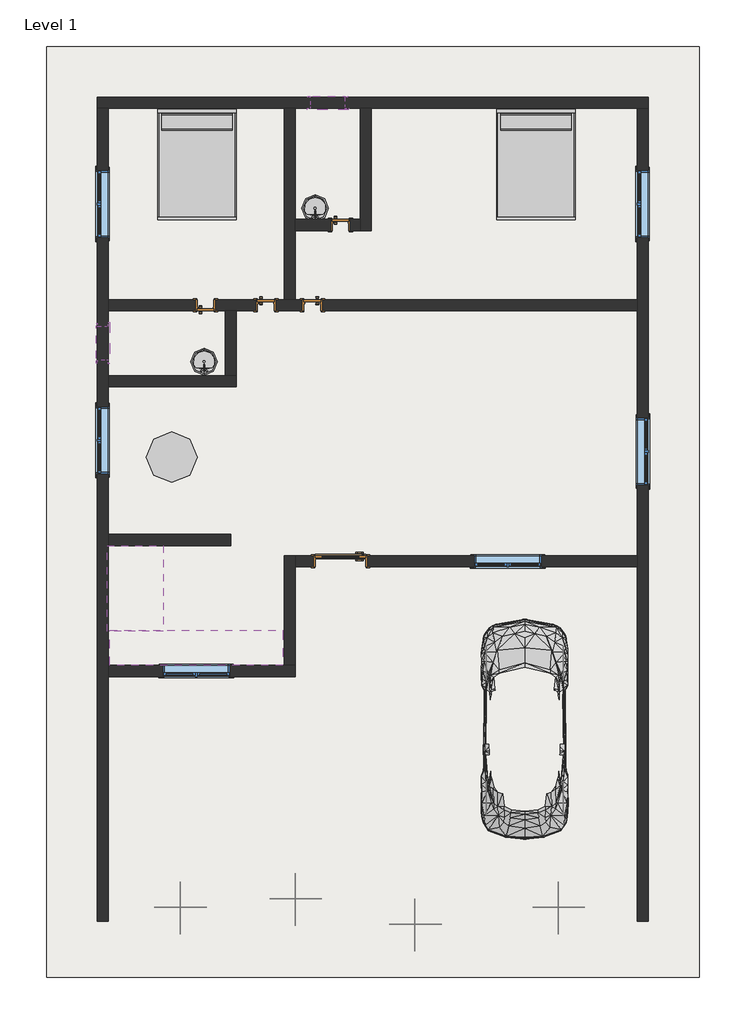
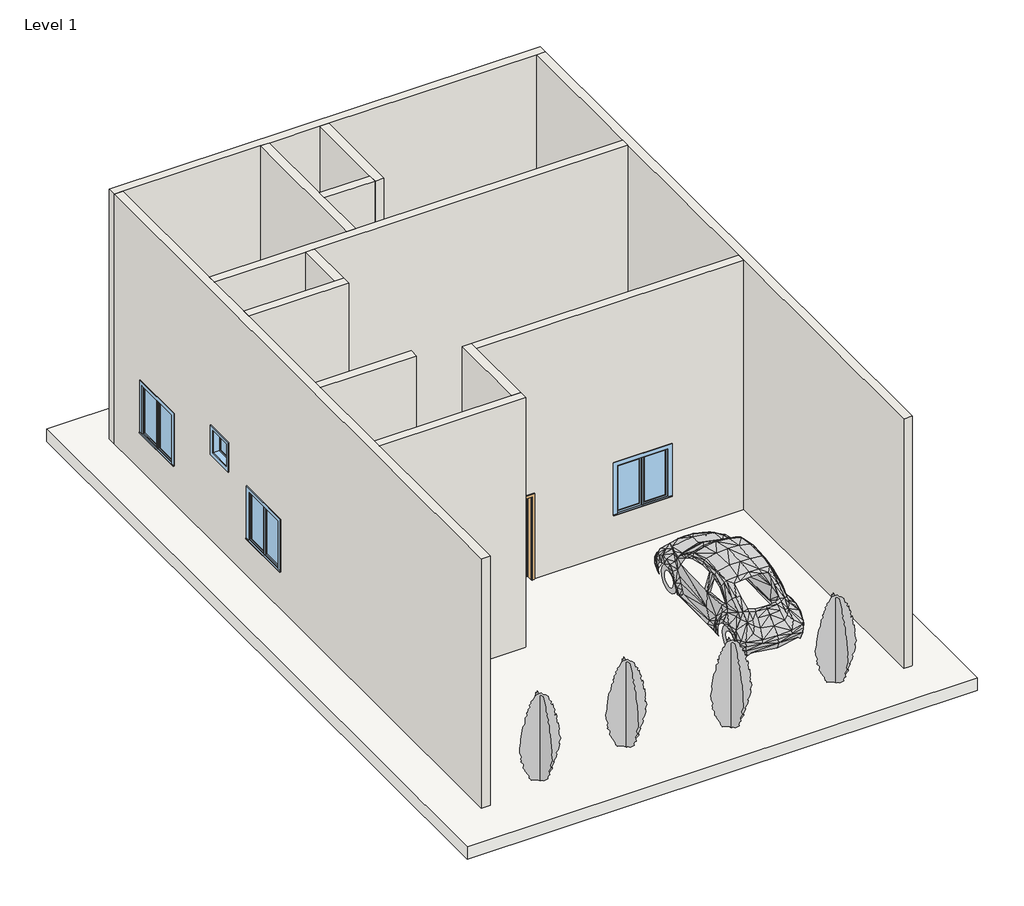
# One storey, incomplete: 13 walls, 8 windows, 5 doors, 5 furniture elements, 4 geographic elements, 2 flow terminals, 1 proxy, 1 slab.
"""IFC4 building model written with IfcOpenShell, lengths in millimetres."""

from ifc_helpers import new_model, si_unit, frame, origin, origin_with_axes, place, context, project, spatial, polyline, outline, extrude, faceted_brep, transform, mapped, element, save
from components import rpc_beetle_rpc_beetle_3ce7ba48, door_1768e003, door_5a382651, door_6ef897ee, door_21b72c96, door_b2d2822a, flow_terminal_d49f872f, furniture_096e7f55, furniture_ac307b45, furniture_905aceb5, furniture_cbbb8910, rpc_tree_conifer_chinese_juniper_7_1b9786cd, window_0862ab64, window_e41d21a6

model = new_model("IFC4")

# Units and contexts
model_context = context("Model", 3, world=origin())
ifc_project = project(units=[si_unit("LENGTHUNIT", "METRE", prefix="MILLI")], contexts=[model_context])

# Site, building, storey
site = spatial("IfcSite", under=ifc_project)
building = spatial("IfcBuilding", under=site)
storey = spatial("IfcBuildingStorey", under=building, Name="Level 1", Elevation=0.0)

# Proxy
placement = place(None, origin())
rpc_beetle_rpc_beetle_shape = rpc_beetle_rpc_beetle_3ce7ba48(model_context)
element("IfcBuildingElementProxy", 1, Name="RPC Beetle : RPC Beetle", ObjectType="RPC Beetle : RPC Beetle", at=placement, inside=storey, context=model_context, shape_type="MappedRepresentation", body=[
    mapped(rpc_beetle_rpc_beetle_shape, transform((-1661.472393, 1425.4293124, 0.0), x_axis=(1.0, 0.0, 0.0), y_axis=(0.0, 1.0, 0.0), z_axis=(0.0, 0.0, 1.0))),
])

# Doors
door_shape = door_1768e003(model_context)
element("IfcDoor", 2, ObjectType="36\" x 80\"", at=placement, inside=storey, context=model_context, shape_type="MappedRepresentation", body=[
    mapped(door_shape, transform((-4988.872393, 5695.8043124, 0.0), x_axis=(1.0, 0.0, 0.0), y_axis=(0.0, 1.0, 0.0), z_axis=(0.0, 0.0, 1.0))),
])
door_2_shape = door_5a382651(model_context)
element("IfcDoor", 3, ObjectType="Door-Interior-Single-5_Panel_Vert-Wood : 12\" x 80\"", at=placement, inside=storey, context=model_context, shape_type="MappedRepresentation", body=[
    mapped(door_2_shape, transform((-6335.072393, 10318.6043124, 0.0), x_axis=(1.0, 0.0, 0.0), y_axis=(0.0, 1.0, 0.0), z_axis=(0.0, 0.0, 1.0))),
])
door_3_shape = door_6ef897ee(model_context)
element("IfcDoor", 4, ObjectType="Door-Interior-Single-5_Panel_Vert-Wood : 12\" x 80\"", at=placement, inside=storey, context=model_context, shape_type="MappedRepresentation", body=[
    mapped(door_3_shape, transform((-5496.872393, 10318.6043124, 0.0), x_axis=(-1.0, 0.0, 0.0), y_axis=(0.0, -1.0, 0.0), z_axis=(0.0, 0.0, 1.0))),
])
door_4_shape = door_21b72c96(model_context)
element("IfcDoor", 5, ObjectType="Door-Interior-Single-Flush_Panel-Wood : 12\" x 80\"", at=placement, inside=storey, context=model_context, shape_type="MappedRepresentation", body=[
    mapped(door_4_shape, transform((-7427.272393, 10312.2543124, 0.0), x_axis=(1.0, 0.0, 0.0), y_axis=(0.0, 1.0, 0.0), z_axis=(0.0, 0.0, 1.0))),
])
door_5_shape = door_b2d2822a(model_context)
element("IfcDoor", 6, ObjectType="Door-Interior-Single-Flush_Panel-Wood : 12\" x 80\"", at=placement, inside=storey, context=model_context, shape_type="MappedRepresentation", body=[
    mapped(door_5_shape, transform((-4988.872393, 11766.4043124, 0.0), x_axis=(1.0, 0.0, 0.0), y_axis=(0.0, 1.0, 0.0), z_axis=(0.0, 0.0, 1.0))),
])

# Flow terminals
flow_terminal_shape = flow_terminal_d49f872f(model_context)
element("IfcFlowTerminal", 7, ObjectType="Sink Vanity-Round : 19\" x 19\"", at=placement, inside=storey, context=model_context, shape_type="MappedRepresentation", body=[
    mapped(flow_terminal_shape, transform((-7356.0206524, 9381.7686876, 0.0), x_axis=(-1.0000000000000004, 0.0, 0.0), y_axis=(0.0, -1.0000000000000004, 0.0), z_axis=(0.0, 0.0, 1.0))),
])
element("IfcFlowTerminal", 8, ObjectType="Sink Vanity-Round : 19\" x 19\"", at=placement, inside=storey, context=model_context, shape_type="MappedRepresentation", body=[
    mapped(flow_terminal_shape, transform((-5349.4206524, 12154.1555452, 0.0), x_axis=(-1.0, 0.0, 0.0), y_axis=(0.0, -1.0, 0.0), z_axis=(0.0, 0.0, 1.0))),
])

# Furniture
furniture_shape = furniture_096e7f55(model_context)
element("IfcFurniture", 9, ObjectType="Bed-Shaker : Double 56\" x 78\"", at=placement, inside=storey, context=model_context, shape_type="MappedRepresentation", body=[
    mapped(furniture_shape, transform((-7560.622393, 13846.0293124, 0.0), x_axis=(1.0, 0.0, 0.0), y_axis=(0.0, 1.0, 0.0), z_axis=(0.0, 0.0, 1.0))),
])
element("IfcFurniture", 10, ObjectType="Bed-Shaker : Double 56\" x 78\"", at=placement, inside=storey, context=model_context, shape_type="MappedRepresentation", body=[
    mapped(furniture_shape, transform((-1439.222393, 13846.0293124, 0.0), x_axis=(1.0, 0.0, 0.0), y_axis=(0.0, 1.0, 0.0), z_axis=(0.0, 0.0, 1.0))),
])
furniture_2_shape = furniture_ac307b45(model_context)
element("IfcFurniture", 11, ObjectType="Counter Top-Island : 48\" Depth", at=placement, inside=storey, context=model_context, shape_type="MappedRepresentation", body=[
    mapped(furniture_2_shape, transform((-9179.872393, 5629.4416075, 914.4), x_axis=(0.0, 1.0000000000000002, 0.0), y_axis=(-1.0000000000000002, 0.0, 0.0), z_axis=(0.0, 0.0, 1.0))),
])
furniture_3_shape = furniture_905aceb5(model_context)
element("IfcFurniture", 12, ObjectType="Table-Dining Round w Chairs : 36\" Diameter", at=placement, inside=storey, context=model_context, shape_type="MappedRepresentation", body=[
    mapped(furniture_3_shape, transform((-8140.5543602, 7757.108001, 0.0), x_axis=(1.0, 0.0, 0.0), y_axis=(0.0, 1.0, 0.0), z_axis=(0.0, 0.0, 1.0))),
])
furniture_4_shape = furniture_cbbb8910(model_context)
element("IfcFurniture", 13, ObjectType="Vanity Counter Top w Square Sink Hole : 24\" Depth", at=placement, inside=storey, context=model_context, shape_type="MappedRepresentation", body=[
    mapped(furniture_4_shape, transform((-7885.7560093, 4448.0293124, 914.4), x_axis=(1.0, 0.0, 0.0), y_axis=(0.0, 1.0, 0.0), z_axis=(0.0, 0.0, 1.0))),
])

# Geographic elements
rpc_tree_conifer_chinese_juniper_7_shape = rpc_tree_conifer_chinese_juniper_7_1b9786cd(model_context)
element("IfcGeographicElement", 14, ObjectType="RPC Tree - Conifer : Chinese Juniper - 7'", at=placement, inside=storey, context=model_context, shape_type="MappedRepresentation", body=[
    mapped(rpc_tree_conifer_chinese_juniper_7_shape, transform((-1052.0690641, -555.7706876, 0.0), x_axis=(1.0, 0.0, 0.0), y_axis=(0.0, 1.0, 0.0), z_axis=(0.0, 0.0, 1.0))),
])
element("IfcGeographicElement", 15, ObjectType="RPC Tree - Conifer : Chinese Juniper - 7'", at=placement, inside=storey, context=model_context, shape_type="MappedRepresentation", body=[
    mapped(rpc_tree_conifer_chinese_juniper_7_shape, transform((-3642.8690641, -860.5706876, 0.0), x_axis=(1.0, 0.0, 0.0), y_axis=(0.0, 1.0, 0.0), z_axis=(0.0, 0.0, 1.0))),
])
element("IfcGeographicElement", 16, ObjectType="RPC Tree - Conifer : Chinese Juniper - 7'", at=placement, inside=storey, context=model_context, shape_type="MappedRepresentation", body=[
    mapped(rpc_tree_conifer_chinese_juniper_7_shape, transform((-7884.6690641, -555.7706876, 0.0), x_axis=(1.0, 0.0, 0.0), y_axis=(0.0, 1.0, 0.0), z_axis=(0.0, 0.0, 1.0))),
])
element("IfcGeographicElement", 17, ObjectType="RPC Tree - Conifer : Chinese Juniper - 7'", at=placement, inside=storey, context=model_context, shape_type="MappedRepresentation", body=[
    mapped(rpc_tree_conifer_chinese_juniper_7_shape, transform((-5801.8690641, -403.3706876, 0.0), x_axis=(1.0, 0.0, 0.0), y_axis=(0.0, 1.0, 0.0), z_axis=(0.0, 0.0, 1.0))),
])

# Slab
element("IfcSlab", 18, ObjectType="Generic - 12\"", at=placement, inside=storey, context=model_context, shape_type="SweptSolid", body=[
    extrude(outline(polyline([(-10297.472393, 14989.0293124), (1488.127607, 14989.0293124), (1488.127607, -1825.7706876), (-10297.472393, -1825.7706876), (-10297.472393, 14989.0293124)])), frame((0.0, 0.0, -304.8), z_axis=(0.0, 0.0, 1.0), x_axis=(1.0, 0.0, 0.0)), (0.0, 0.0, 1.0), 304.8),
])

# Walls
element("IfcWall", 19, ObjectType="Generic - 8\"", at=placement, inside=storey, context=model_context, shape_type="Brep", body=[
    faceted_brep([(-9383.072393, 13871.4293124, 0.0), (-9179.872393, 13871.4293124, 0.0), (-6004.872393, 13871.4293124, 0.0), (-5801.672393, 13871.4293124, 0.0), (-4633.272393, 13871.4293124, 0.0), (-4430.072393, 13871.4293124, 0.0), (370.527607, 13871.4293124, 0.0), (573.727607, 13871.4293124, 0.0), (573.727607, 13871.4293124, 6096.0), (370.527607, 13871.4293124, 6096.0), (-4430.072393, 13871.4293124, 6096.0), (-4633.272393, 13871.4293124, 6096.0), (-5801.672393, 13871.4293124, 6096.0), (-6004.872393, 13871.4293124, 6096.0), (-9179.872393, 13871.4293124, 6096.0), (-9383.072393, 13871.4293124, 6096.0), (-5522.272393, 13871.4293124, 2768.6), (-4912.672393, 13871.4293124, 2768.6), (-4912.672393, 13871.4293124, 2159.0), (-5522.272393, 13871.4293124, 2159.0), (-9383.072393, 14074.6293124, 0.0), (-9383.072393, 14074.6293124, 6096.0), (573.727607, 14074.6293124, 6096.0), (573.727607, 14074.6293124, 0.0), (-5522.272393, 14074.6293124, 2768.6), (-5522.272393, 14074.6293124, 2159.0), (-4912.672393, 14074.6293124, 2159.0), (-4912.672393, 14074.6293124, 2768.6)], [[[0, 1, 2, 3, 4, 5, 6, 7, 8, 9, 10, 11, 12, 13, 14, 15], [16, 17, 18, 19]], [[20, 21, 22, 23], [24, 25, 26, 27]], [[7, 6, 5, 4, 3, 2, 1, 0, 20, 23]], [[15, 14, 13, 12, 11, 10, 9, 8, 22, 21]], [[8, 7, 23, 22]], [[0, 15, 21, 20]], [[25, 24, 16, 19]], [[26, 25, 19, 18]], [[27, 26, 18, 17]], [[24, 27, 17, 16]]]),
])
element("IfcWall", 20, ObjectType="Generic - 8\"", at=placement, inside=storey, context=model_context, shape_type="Brep", body=[
    faceted_brep([(370.527607, 13871.4293124, 0.0), (370.527607, 10417.0293124, 0.0), (370.527607, 10213.8293124, 0.0), (370.527607, 5794.2293124, 0.0), (370.527607, 5591.0293124, 0.0), (370.527607, -809.7706876, 0.0), (370.527607, -809.7706876, 6096.0), (370.527607, 5591.0293124, 6096.0), (370.527607, 5794.2293124, 6096.0), (370.527607, 10213.8293124, 6096.0), (370.527607, 10417.0293124, 6096.0), (370.527607, 13871.4293124, 6096.0), (370.527607, 12753.8293124, 2133.6), (370.527607, 11534.6293124, 2133.6), (370.527607, 11534.6293124, 914.4), (370.527607, 12753.8293124, 914.4), (370.527607, 7064.2293124, 2133.6), (370.527607, 7064.2293124, 914.4), (370.527607, 8283.4293124, 914.4), (370.527607, 8283.4293124, 2133.6), (573.727607, 13871.4293124, 0.0), (573.727607, 13871.4293124, 6096.0), (573.727607, -809.7706876, 6096.0), (573.727607, -809.7706876, 0.0), (573.727607, 12753.8293124, 2133.6), (573.727607, 12753.8293124, 914.4), (573.727607, 11534.6293124, 914.4), (573.727607, 11534.6293124, 2133.6), (573.727607, 7064.2293124, 2133.6), (573.727607, 8283.4293124, 2133.6), (573.727607, 8283.4293124, 914.4), (573.727607, 7064.2293124, 914.4)], [[[0, 1, 2, 3, 4, 5, 6, 7, 8, 9, 10, 11], [12, 13, 14, 15], [16, 17, 18, 19]], [[20, 21, 22, 23], [24, 25, 26, 27], [28, 29, 30, 31]], [[5, 4, 3, 2, 1, 0, 20, 23]], [[6, 5, 23, 22]], [[11, 10, 9, 8, 7, 6, 22, 21]], [[0, 11, 21, 20]], [[25, 24, 12, 15]], [[26, 25, 15, 14]], [[27, 26, 14, 13]], [[24, 27, 13, 12]], [[17, 16, 28, 31]], [[18, 17, 31, 30]], [[19, 18, 30, 29]], [[16, 19, 29, 28]]]),
])
element("IfcWall", 21, ObjectType="Generic - 8\"", at=placement, inside=storey, context=model_context, shape_type="Brep", body=[
    faceted_brep([(-9179.872393, -809.7706876, 0.0), (-9179.872393, 3609.8293124, 0.0), (-9179.872393, 3813.0293124, 0.0), (-9179.872393, 5972.0293124, 0.0), (-9179.872393, 6175.2293124, 0.0), (-9179.872393, 8842.2293124, 0.0), (-9179.872393, 9045.4293124, 0.0), (-9179.872393, 10213.8293124, 0.0), (-9179.872393, 10417.0293124, 0.0), (-9179.872393, 13871.4293124, 0.0), (-9179.872393, 13871.4293124, 6096.0), (-9179.872393, 10417.0293124, 6096.0), (-9179.872393, 10213.8293124, 6096.0), (-9179.872393, 9045.4293124, 6096.0), (-9179.872393, 8842.2293124, 6096.0), (-9179.872393, 6175.2293124, 6096.0), (-9179.872393, 5972.0293124, 6096.0), (-9179.872393, 3813.0293124, 6096.0), (-9179.872393, 3609.8293124, 6096.0), (-9179.872393, -809.7706876, 6096.0), (-9179.872393, 12753.8293124, 2133.6), (-9179.872393, 12753.8293124, 914.4), (-9179.872393, 11534.6293124, 914.4), (-9179.872393, 11534.6293124, 2133.6), (-9179.872393, 8486.6293124, 2133.6), (-9179.872393, 8486.6293124, 914.4), (-9179.872393, 7267.4293124, 914.4), (-9179.872393, 7267.4293124, 2133.6), (-9179.872393, 9324.8293124, 2768.6), (-9179.872393, 9934.4293124, 2768.6), (-9179.872393, 9934.4293124, 2159.0), (-9179.872393, 9324.8293124, 2159.0), (-9383.072393, -809.7706876, 0.0), (-9383.072393, -809.7706876, 6096.0), (-9383.072393, 13871.4293124, 6096.0), (-9383.072393, 13871.4293124, 0.0), (-9383.072393, 12753.8293124, 2133.6), (-9383.072393, 11534.6293124, 2133.6), (-9383.072393, 11534.6293124, 914.4), (-9383.072393, 12753.8293124, 914.4), (-9383.072393, 8486.6293124, 2133.6), (-9383.072393, 7267.4293124, 2133.6), (-9383.072393, 7267.4293124, 914.4), (-9383.072393, 8486.6293124, 914.4), (-9383.072393, 9324.8293124, 2768.6), (-9383.072393, 9324.8293124, 2159.0), (-9383.072393, 9934.4293124, 2159.0), (-9383.072393, 9934.4293124, 2768.6)], [[[0, 1, 2, 3, 4, 5, 6, 7, 8, 9, 10, 11, 12, 13, 14, 15, 16, 17, 18, 19], [20, 21, 22, 23], [24, 25, 26, 27], [28, 29, 30, 31]], [[32, 33, 34, 35], [36, 37, 38, 39], [40, 41, 42, 43], [44, 45, 46, 47]], [[9, 8, 7, 6, 5, 4, 3, 2, 1, 0, 32, 35]], [[19, 18, 17, 16, 15, 14, 13, 12, 11, 10, 34, 33]], [[0, 19, 33, 32]], [[10, 9, 35, 34]], [[21, 20, 36, 39]], [[22, 21, 39, 38]], [[23, 22, 38, 37]], [[20, 23, 37, 36]], [[25, 24, 40, 43]], [[26, 25, 43, 42]], [[27, 26, 42, 41]], [[24, 27, 41, 40]], [[45, 44, 28, 31]], [[46, 45, 31, 30]], [[47, 46, 30, 29]], [[44, 47, 29, 28]]]),
])
element("IfcWall", 22, ObjectType="Generic - 8\"", at=placement, inside=storey, context=model_context, shape_type="Brep", body=[
    faceted_brep([(370.527607, 10213.8293124, 6096.0), (-6868.472393, 10213.8293124, 6096.0), (-7071.672393, 10213.8293124, 6096.0), (-9179.872393, 10213.8293124, 6096.0), (-9179.872393, 10213.8293124, 0.0), (-7605.072393, 10213.8293124, 0.0), (-7605.072393, 10213.8293124, 2057.4), (-7249.472393, 10213.8293124, 2057.4), (-7249.472393, 10213.8293124, 0.0), (-7071.672393, 10213.8293124, 0.0), (-6868.472393, 10213.8293124, 0.0), (-6512.872393, 10213.8293124, 0.0), (-6512.872393, 10213.8293124, 2057.4), (-6157.272393, 10213.8293124, 2057.4), (-6157.272393, 10213.8293124, 0.0), (-5674.672393, 10213.8293124, 0.0), (-5674.672393, 10213.8293124, 2057.4), (-5319.072393, 10213.8293124, 2057.4), (-5319.072393, 10213.8293124, 0.0), (370.527607, 10213.8293124, 0.0), (-9179.872393, 10417.0293124, 6096.0), (-6004.872393, 10417.0293124, 6096.0), (-5801.672393, 10417.0293124, 6096.0), (370.527607, 10417.0293124, 6096.0), (370.527607, 10417.0293124, 0.0), (-5319.072393, 10417.0293124, 0.0), (-5319.072393, 10417.0293124, 2057.4), (-5674.672393, 10417.0293124, 2057.4), (-5674.672393, 10417.0293124, 0.0), (-5801.672393, 10417.0293124, 0.0), (-6004.872393, 10417.0293124, 0.0), (-6157.272393, 10417.0293124, 0.0), (-6157.272393, 10417.0293124, 2057.4), (-6512.872393, 10417.0293124, 2057.4), (-6512.872393, 10417.0293124, 0.0), (-7249.472393, 10417.0293124, 0.0), (-7249.472393, 10417.0293124, 2057.4), (-7605.072393, 10417.0293124, 2057.4), (-7605.072393, 10417.0293124, 0.0), (-9179.872393, 10417.0293124, 0.0)], [[[0, 1, 2, 3, 4, 5, 6, 7, 8, 9, 10, 11, 12, 13, 14, 15, 16, 17, 18, 19]], [[20, 21, 22, 23, 24, 25, 26, 27, 28, 29, 30, 31, 32, 33, 34, 35, 36, 37, 38, 39]], [[4, 39, 38, 5]], [[24, 19, 18, 25]], [[14, 31, 30, 29, 28, 15]], [[34, 11, 10, 9, 8, 35]], [[3, 2, 1, 0, 23, 22, 21, 20]], [[0, 19, 24, 23]], [[4, 3, 20, 39]], [[13, 32, 31, 14]], [[32, 13, 12, 33]], [[33, 12, 11, 34]], [[27, 16, 15, 28]], [[16, 27, 26, 17]], [[17, 26, 25, 18]], [[7, 36, 35, 8]], [[36, 7, 6, 37]], [[37, 6, 5, 38]]]),
])
element("IfcWall", 23, ObjectType="Generic - 8\"", at=placement, inside=storey, context=model_context, shape_type="SweptSolid", body=[
    extrude(outline(polyline([(6096.0, -4633.272393), (6096.0, -5801.672393), (0.0, -5801.672393), (0.0, -5166.672393), (2057.4, -5166.672393), (2057.4, -4811.072393), (0.0, -4811.072393), (0.0, -4633.272393), (6096.0, -4633.272393)])), frame((0.0, 11661.6293124, 0.0), z_axis=(0.0, 1.0, 0.0), x_axis=(0.0, 0.0, 1.0)), (0.0, 0.0, 1.0), 203.2),
])
element("IfcWall", 24, ObjectType="Generic - 8\"", at=placement, inside=storey, context=model_context, shape_type="Brep", body=[
    faceted_brep([(-4430.072393, 11661.6293124, 0.0), (-4430.072393, 13871.4293124, 0.0), (-4430.072393, 13871.4293124, 6096.0), (-4430.072393, 11661.6293124, 6096.0), (-4633.272393, 11661.6293124, 0.0), (-4633.272393, 11661.6293124, 6096.0), (-4633.272393, 11864.8293124, 6096.0), (-4633.272393, 13871.4293124, 6096.0), (-4633.272393, 13871.4293124, 0.0), (-4633.272393, 11864.8293124, 0.0)], [[[0, 1, 2, 3]], [[4, 5, 6, 7, 8, 9]], [[1, 0, 4, 9, 8]], [[3, 2, 7, 6, 5]], [[0, 3, 5, 4]], [[2, 1, 8, 7]]]),
])
element("IfcWall", 25, ObjectType="Generic - 8\"", at=placement, inside=storey, context=model_context, shape_type="Brep", body=[
    faceted_brep([(-5801.672393, 13871.4293124, 0.0), (-5801.672393, 13871.4293124, 6096.0), (-5801.672393, 11864.8293124, 6096.0), (-5801.672393, 11661.6293124, 6096.0), (-5801.672393, 10417.0293124, 6096.0), (-5801.672393, 10417.0293124, 0.0), (-5801.672393, 11661.6293124, 0.0), (-5801.672393, 11864.8293124, 0.0), (-6004.872393, 13871.4293124, 6096.0), (-6004.872393, 13871.4293124, 0.0), (-6004.872393, 10417.0293124, 0.0), (-6004.872393, 10417.0293124, 6096.0)], [[[0, 1, 2, 3, 4, 5, 6, 7]], [[8, 9, 10, 11]], [[9, 0, 7, 6, 5, 10]], [[1, 8, 11, 4, 3, 2]], [[1, 0, 9, 8]], [[5, 4, 11, 10]]]),
])
element("IfcWall", 26, ObjectType="Generic - 8\"", at=placement, inside=storey, context=model_context, shape_type="Brep", body=[
    faceted_brep([(-9179.872393, 8842.2293124, 0.0), (-6868.472393, 8842.2293124, 0.0), (-6868.472393, 8842.2293124, 6096.0), (-9179.872393, 8842.2293124, 6096.0), (-9179.872393, 9045.4293124, 0.0), (-9179.872393, 9045.4293124, 6096.0), (-7071.672393, 9045.4293124, 6096.0), (-6868.472393, 9045.4293124, 6096.0), (-6868.472393, 9045.4293124, 0.0), (-7071.672393, 9045.4293124, 0.0)], [[[0, 1, 2, 3]], [[4, 5, 6, 7, 8, 9]], [[1, 0, 4, 9, 8]], [[3, 2, 7, 6, 5]], [[0, 3, 5, 4]], [[2, 1, 8, 7]]]),
])
element("IfcWall", 27, ObjectType="Generic - 8\"", at=placement, inside=storey, context=model_context, shape_type="SweptSolid", body=[
    extrude(outline(polyline([(-6868.472393, 10213.8293124), (-6868.472393, 9045.4293124), (-7071.672393, 9045.4293124), (-7071.672393, 10213.8293124), (-6868.472393, 10213.8293124)])), origin_with_axes(), (0.0, 0.0, 1.0), 6096.0),
])
element("IfcWall", 28, ObjectType="Generic - 8\"", at=placement, inside=storey, context=model_context, shape_type="Brep", body=[
    faceted_brep([(-9179.872393, 3609.8293124, 0.0), (-5801.672393, 3609.8293124, 0.0), (-5801.672393, 3609.8293124, 6096.0), (-9179.872393, 3609.8293124, 6096.0), (-8201.972393, 3609.8293124, 2133.6), (-6982.772393, 3609.8293124, 2133.6), (-6982.772393, 3609.8293124, 914.4), (-8201.972393, 3609.8293124, 914.4), (-9179.872393, 3813.0293124, 0.0), (-9179.872393, 3813.0293124, 6096.0), (-6004.872393, 3813.0293124, 6096.0), (-5801.672393, 3813.0293124, 6096.0), (-5801.672393, 3813.0293124, 0.0), (-6004.872393, 3813.0293124, 0.0), (-8201.972393, 3813.0293124, 2133.6), (-8201.972393, 3813.0293124, 914.4), (-6982.772393, 3813.0293124, 914.4), (-6982.772393, 3813.0293124, 2133.6)], [[[0, 1, 2, 3], [4, 5, 6, 7]], [[8, 9, 10, 11, 12, 13], [14, 15, 16, 17]], [[1, 0, 8, 13, 12]], [[3, 2, 11, 10, 9]], [[0, 3, 9, 8]], [[2, 1, 12, 11]], [[15, 14, 4, 7]], [[16, 15, 7, 6]], [[17, 16, 6, 5]], [[14, 17, 5, 4]]]),
])
element("IfcWall", 29, ObjectType="Generic - 8\"", at=placement, inside=storey, context=model_context, shape_type="SweptSolid", body=[
    extrude(outline(polyline([(-6970.072393, 5972.0293124), (-9179.872393, 5972.0293124), (-9179.872393, 6175.2293124), (-6970.072393, 6175.2293124), (-6970.072393, 5972.0293124)])), origin_with_axes(), (0.0, 0.0, 1.0), 6096.0),
])
element("IfcWall", 30, ObjectType="Generic - 8\"", at=placement, inside=storey, context=model_context, shape_type="Brep", body=[
    faceted_brep([(-5801.672393, 3813.0293124, 0.0), (-5801.672393, 5591.0293124, 0.0), (-5801.672393, 5794.2293124, 0.0), (-5801.672393, 5794.2293124, 6096.0), (-5801.672393, 5591.0293124, 6096.0), (-5801.672393, 3813.0293124, 6096.0), (-6004.872393, 3813.0293124, 0.0), (-6004.872393, 3813.0293124, 6096.0), (-6004.872393, 5794.2293124, 6096.0), (-6004.872393, 5794.2293124, 0.0)], [[[0, 1, 2, 3, 4, 5]], [[6, 7, 8, 9]], [[2, 1, 0, 6, 9]], [[5, 4, 3, 8, 7]], [[3, 2, 9, 8]], [[0, 5, 7, 6]]]),
])
element("IfcWall", 31, ObjectType="Generic - 8\"", at=placement, inside=storey, context=model_context, shape_type="SweptSolid", body=[
    extrude(outline(polyline([(6096.0, 370.527607), (6096.0, -5801.672393), (0.0, -5801.672393), (0.0, -5471.472393), (2057.4, -5471.472393), (2057.4, -4506.272393), (0.0, -4506.272393), (0.0, 370.527607), (6096.0, 370.527607)]), holes=[polyline([(2133.6, -2575.872393), (2133.6, -1356.672393), (914.4, -1356.672393), (914.4, -2575.872393), (2133.6, -2575.872393)])]), frame((0.0, 5591.0293124, 0.0), z_axis=(0.0, 1.0, 0.0), x_axis=(0.0, 0.0, 1.0)), (0.0, 0.0, 1.0), 203.2),
])

# Windows
window_shape = window_0862ab64(model_context)
element("IfcWindow", 32, ObjectType="Casement Dbl with Trim : 48\" x 48\"", at=placement, inside=storey, context=model_context, shape_type="MappedRepresentation", body=[
    mapped(window_shape, transform((491.177607, 12144.2293124, 0.0), x_axis=(0.0, 1.0, 0.0), y_axis=(-1.0, 0.0, 0.0), z_axis=(0.0, 0.0, 1.0))),
])
element("IfcWindow", 33, ObjectType="Casement Dbl with Trim : 48\" x 48\"", at=placement, inside=storey, context=model_context, shape_type="MappedRepresentation", body=[
    mapped(window_shape, transform((-9262.422393, 12144.2293124, 0.0), x_axis=(0.0, 1.0, 0.0), y_axis=(-1.0, 0.0, 0.0), z_axis=(0.0, 0.0, 1.0))),
])
element("IfcWindow", 34, ObjectType="Casement Dbl with Trim : 48\" x 48\"", at=placement, inside=storey, context=model_context, shape_type="MappedRepresentation", body=[
    mapped(window_shape, transform((453.077607, 7673.8293124, 0.0), x_axis=(0.0, -1.0, 0.0), y_axis=(1.0, 0.0, 0.0), z_axis=(0.0, 0.0, 1.0))),
])
element("IfcWindow", 35, ObjectType="Casement Dbl with Trim : 48\" x 48\"", at=placement, inside=storey, context=model_context, shape_type="MappedRepresentation", body=[
    mapped(window_shape, transform((-1966.272393, 5711.6793124, 0.0), x_axis=(-1.0, 0.0, 0.0), y_axis=(0.0, -1.0, 0.0), z_axis=(0.0, 0.0, 1.0))),
])
element("IfcWindow", 36, ObjectType="Casement Dbl with Trim : 48\" x 48\"", at=placement, inside=storey, context=model_context, shape_type="MappedRepresentation", body=[
    mapped(window_shape, transform((-7592.372393, 3730.4793124, 0.0), x_axis=(-1.0, 0.0, 0.0), y_axis=(0.0, -1.0, 0.0), z_axis=(0.0, 0.0, 1.0))),
])
element("IfcWindow", 37, ObjectType="Casement Dbl with Trim : 48\" x 48\"", at=placement, inside=storey, context=model_context, shape_type="MappedRepresentation", body=[
    mapped(window_shape, transform((-9262.422393, 7877.0293124, 0.0), x_axis=(0.0, 1.0, 0.0), y_axis=(-1.0, 0.0, 0.0), z_axis=(0.0, 0.0, 1.0))),
])
window_2_shape = window_e41d21a6(model_context)
element("IfcWindow", 38, ObjectType="Transom with Trim : 24\" x 24\"", at=placement, inside=storey, context=model_context, shape_type="MappedRepresentation", body=[
    mapped(window_2_shape, transform((-9281.472393, 9591.5293124, 0.0), x_axis=(0.0, -1.0, 0.0), y_axis=(1.0, 0.0, 0.0), z_axis=(0.0, 0.0, 1.0))),
])
element("IfcWindow", 39, ObjectType="Transom with Trim : 24\" x 24\"", at=placement, inside=storey, context=model_context, shape_type="MappedRepresentation", body=[
    mapped(window_2_shape, transform((-5255.572393, 13973.0293124, 0.0), x_axis=(-1.0, 0.0, 0.0), y_axis=(0.0, -1.0, 0.0), z_axis=(0.0, 0.0, 1.0))),
])

save(model, "model.ifc")

# Revit data of these elements
# Type "RPC Beetle : RPC Beetle"
#   built-in parameter 1005195 = "RPC-16-0U6E-L4EG-ENH1-J3KF-SVEL-0TX4-C0"
#   Height = 0
# Type "36\" x 80\""
#   Type Mark = "11"
#   Assembly Code = "B2030100"
#   Analytic Construction = "French door, wood frame with single glass"
#   Threshold Offset [instance default] = 0' - 0 1/2"
#   Thickness = 0' - 1 3/8"
#   Thermal Resistance (R) = 1.0696 (h·ft²·°F)/BTU
#   Swing Angle [instance default] = 90.00°
#   Stiles = 0' - 4 3/4"
#   Rough Width = 3' - 2"
#   Rough Height = 6' - 9"
#   Radius = 1' - 8.05625"
#   Lock Rail = 0' - 7 1/8"
#   Height = 6' - 8"
#   Width = 3' - 0"
#   Heat Transfer Coefficient (U) = 0.9350 BTU/(h·ft²·°F)
#   Door Offset [instance default] = 0' - 0"
#   Bottom Rail = 0' - 9 1/2"
#   Threshold [instance default] = yes
#   Function = 1
#   Exterior Trim [instance default] = yes
#   Trim Material = Cherry
#   Threshold Material = Cherry
#   Panel Material = Cherry
#   Glazing = Glass
#   Frame Material = Cherry
#   Door Handle Material = Aluminum
#   Visual Light Transmittance = 0
#   Solar Heat Gain Coefficient = 0
#   Wall Closure = (empty or 0)
#   Construction Type = (empty or 0)
# Type "Door-Interior-Single-5_Panel_Vert-Wood : 12\" x 80\""
#   Type Mark = "8"
#   Assembly Code = "C1020300"
#   Analytic Construction = "Wooden"
#   Top Rail = 0' - 4 11/16"
#   Thickness = 0' - 1 3/8"
#   Thermal Resistance (R) = 2.5876 (h·ft²·°F)/BTU
#   Swing Angle [instance default] = 90.00°
#   Stiles = 0' - 2 3/8"
#   Rough Width = 1' - 2"
#   Rough Height = 6' - 9"
#   Intermediate Rail = 0' - 4 1/2"
#   Height = 6' - 8"
#   Width = 1' - 0"
#   Heat Transfer Coefficient (U) = 0.3865 BTU/(h·ft²·°F)
#   Bottom Rail = 0' - 9 1/8"
#   Trim Material = Cherry
#   Panel Material = Cherry
#   Frame Material = Cherry
#   Door Handle Material = Aluminum
#   Visual Light Transmittance = 0
#   Solar Heat Gain Coefficient = 0
#   Wall Closure = (empty or 0)
#   Function = (empty or 0)
# Type "Door-Interior-Single-Flush_Panel-Wood : 12\" x 80\""
#   Type Mark = "9"
#   Assembly Code = "C1020300"
#   Analytic Construction = "Wooden"
#   Thickness = 0' - 1 3/8"
#   Thermal Resistance (R) = 2.5876 (h·ft²·°F)/BTU
#   Swing Angle [instance default] = 90.00°
#   Rough Width = 1' - 2"
#   Rough Height = 6' - 9"
#   Height = 6' - 8"
#   Width = 1' - 0"
#   Heat Transfer Coefficient (U) = 0.3865 BTU/(h·ft²·°F)
#   Trim Material = Cherry
#   Panel Material = Cherry
#   Frame Material = Cherry
#   Door Handle Material = Aluminum
#   Visual Light Transmittance = 0
#   Solar Heat Gain Coefficient = 0
#   Wall Closure = (empty or 0)
#   Function = (empty or 0)
# Type "Sink Vanity-Round : 19\" x 19\""
#   Assembly Code = "D2010400"
#   Top Of Counter = 2' - 7"
#   Basin Material = Porcelain, Linen
#   Faucet Material = Steel, Polished
#   Default Elevation = 0
# Type "Bed-Shaker : Double 56\" x 78\""
#   Assembly Code = "E2020200"
#   Length = 6' - 6"
#   Width = 4' - 8"
#   Frame Material = Birch
#   Mattress Material = Linen, White
#   Default Elevation = 0
# Type "Counter Top-Island : 48\" Depth"
#   Assembly Code = "C1030400"
#   Counter Thickness = 0' - 1 1/2"
#   Depth [instance default] = 4' - 2"
#   Height = 3' - 0"
#   Length [instance default] = 8' - 0"
#   Counter Top Material = none
#   Default Elevation = 0
# Type "Table-Dining Round w Chairs : 36\" Diameter"
#   Assembly Code = "E2020200"
#   Radius = 1' - 6"
#   Diameter = 3' - 0"
#   Height = 2' - 6"
#   Chairs = 4
#   Base Material = Pine
#   Top Material = Laminate, Linen, Matte
#   Default Elevation = 0
# Type "Vanity Counter Top w Square Sink Hole : 24\" Depth"
#   Assembly Code = "C1030400"
#   Counter Thickness = 0' - 1 1/2"
#   Depth = 2' - 1"
#   Height = 2' - 7"
#   Length [instance default] = 4' - 0"
#   Sink Location [instance default] = 2' - 0"
#   Sink Location To Wall [instance default] = 0' - 4 1/2"
#   Sink Opening Depth [instance default] = 1' - 5 1/2"
#   Sink Opening Width [instance default] = 1' - 8"
#   Counter Top Material = none
#   Default Elevation = 0
# Type "RPC Tree - Conifer : Chinese Juniper - 7'"
#   built-in parameter 1005198 = "{2, 15},{39, RPC-16-FUM3-UUQ0-UBF0-N000-ST1L-LVER-AU},{1, 0},{1, 0},{2, 13},{1, 8},{5, Color},{1, 0},{1, 0},{3, 0.8},{3, 0.8},{3, 0.8},{1, 8},{7, BBoxMin},{1, 0},{1, 0},{1, 0},{1, 0},{1, 0},{1, 8},{7, BBoxMax},{1, 0},{1, 0},{1, 0},{1, 0},{1, 0},{2, 11},{9, RPCTypeId},{1, 0},{1, 0},{39, RPC-16-FUM3-UUQ0-UBF0-N000-ST1L-LVER-AU},{1, 6},{14, RPCPlantHeight},{1, 0},{1, 0},{1, 7},{2, 11},{7, keyword},{1, 0},{1, 0},{34, :RPCs:Trees [General]:Geometry:RPC},{2, 11},{8, category},{1, 0},{1, 0},{15, Trees [General]},{2, 11},{12, LocalizedUID},{1, 0},{1, 0},{15, Chinese Juniper},{2, 14},{6, Height},{1, 0},{1, 0},{1, 7},{1, 2},{16, Cast Reflections},{1, 0},{1, 0},{1, 0},{1, 2},{12, Cast Shadows},{1, 0},{1, 0},{1, 1},{1, 2},{9, Lock View},{1, 0},{1, 0},{1, 0},{1, 4},{5, ViewC},{1, 0},{1, 0},{1, 0},{21, assetlibrary_base.fbx},{1, 5},"
#   built-in parameter 1005195 = "RPC-16-FUM3-UUQ0-UBF0-N000-ST1L-LVER-AU"
#   Type Comments = "Chinese Juniper"
#   Assembly Code = "G2050500"
#   Height = 7' - 0"
#   Description = (empty or 0)
#   Default Elevation = 0
# Type "Generic - 12\""
#   Assembly Code = "B1010"
#   Function = 0
#   Layers, outside or top first: 1' - 0" no material (function 1)
# Type "Generic - 8\""
#   Assembly Code = "B2010"
#   Layers, outside or top first: 0' - 8" no material (function 1)
# Type "Casement Dbl with Trim : 48\" x 48\""
#   Type Mark = "10"
#   Construction Type Id = "GSP4R"
#   Assembly Code = "B2020100"
#   Analytic Construction = "1/8 in Pilkington single glazing"
#   Visual Light Transmittance = 0.9
#   Solar Heat Gain Coefficient = 0.78
#   Heat Transfer Coefficient (U) = 0.6496 BTU/(h·ft²·°F)
#   Height = 4' - 0"
#   Default Sill Height = 3' - 0"
#   Trim Projection - Ext. = 0' - 0 1/2"
#   Trim Projection - Int. = 0' - 0 3/4"
#   Trim Width - Exterior = 0' - 3 1/2"
#   Trim Width - Interior = 0' - 3 1/2"
#   Width = 4' - 0"
#   Window Inset = 0' - 0 3/4"
#   Define Thermal Properties by = 1
#   Glass Pane Material = Glass
#   Sash Material = Sash
#   Trim Exterior Material = Trim
#   Trim Interior Material = Trim
#   Wall Closure = (empty or 0)
# Type "Transom with Trim : 24\" x 24\""
#   Type Mark = "13"
#   Construction Type Id = "GSP4R"
#   Assembly Code = "B2020100"
#   Analytic Construction = "1/8 in Pilkington single glazing"
#   Visual Light Transmittance = 0.9
#   Solar Heat Gain Coefficient = 0.78
#   Heat Transfer Coefficient (U) = 0.6496 BTU/(h·ft²·°F)
#   Height = 2' - 0"
#   Default Sill Height = 7' - 1"
#   Trim Projection - Ext. = 0' - 0 1/2"
#   Trim Projection - Int. = 0' - 0 3/4"
#   Trim Width - Exterior = 0' - 3 1/2"
#   Trim Width - Interior = 0' - 3 1/2"
#   Width = 2' - 0"
#   Window Inset = 0' - 0 3/4"
#   Define Thermal Properties by = 1
#   Glass Pane Material = Glass
#   Sash Material = Sash
#   Trim Exterior Material = Trim
#   Trim Interior Material = Trim
#   Wall Closure = (empty or 0)
# Element 1 (IfcBuildingElementProxy, "RPC Beetle : RPC Beetle")
#   Phase Created = New Construction
# Element 2 (IfcDoor, "36\" x 80\"")
#   Threshold Offset = 0' - 0 1/2"
#   Swing Angle = 90.00°
#   Door Offset = 0' - 0"
#   Threshold = yes
#   Exterior Trim = yes
#   Phase Created = New Construction
#   Materials on its faces: "Cherry", "Aluminum", "Glass"
# Elements 3, 4 (IfcDoor, "Door-Interior-Single-5_Panel_Vert-Wood : 12\" x 80\"")
#   Swing Angle = 90.00°
#   Phase Created = New Construction
#   Materials on its faces: "Cherry", "Aluminum"
# Elements 5, 6 (IfcDoor, "Door-Interior-Single-Flush_Panel-Wood : 12\" x 80\"")
#   Swing Angle = 90.00°
#   Phase Created = New Construction
#   Materials on its faces: "Cherry", "Aluminum"
# Element 7 (IfcFlowTerminal, "Sink Vanity-Round : 19\" x 19\"")
#   Mark = "1"
#   Phase Created = New Construction
#   Materials on its faces: "Porcelain, Linen", "Steel, Polished"
# Element 8 (IfcFlowTerminal, "Sink Vanity-Round : 19\" x 19\"")
#   Mark = "2"
#   Phase Created = New Construction
#   Materials on its faces: "Porcelain, Linen", "Steel, Polished"
# Elements 9, 10 (IfcFurniture, "Bed-Shaker : Double 56\" x 78\"")
#   Phase Created = New Construction
#   Materials on its faces: "Birch", "Linen, White"
# Element 11 (IfcFurniture, "Counter Top-Island : 48\" Depth")
#   Length = 5' - 0 3/4"
#   Depth = 3' - 4.02886"
#   Phase Created = New Construction
#   Materials on its faces: "Counter Top"
# Element 12 (IfcFurniture, "Table-Dining Round w Chairs : 36\" Diameter")
#   Phase Created = New Construction
#   Materials on its faces: "Pine", "Laminate, Linen, Matte"
# Element 13 (IfcFurniture, "Vanity Counter Top w Square Sink Hole : 24\" Depth")
#   Sink Opening Width = 1' - 8"
#   Sink Opening Depth = 1' - 5 1/2"
#   Sink Location To Wall = 0' - 4 1/2"
#   Sink Location = 4' - 2.00033"
#   Length = 10' - 3.00033"
#   Phase Created = New Construction
#   Materials on its faces: "Counter Top"
# Elements 14, 15, 16, 17 (IfcGeographicElement, "RPC Tree - Conifer : Chinese Juniper - 7'")
#   Phase Created = New Construction
# Element 18 (IfcSlab, "Generic - 12\"")
#   built-in parameter 1001955 = 1.5708 (stored number, unit not read)
#   Height Offset From Level = 0' - 0"
#   Phase Created = New Construction
#   Materials on its faces: "Default Floor"
# Elements 19, 20, 21, 22, 23, 24, 25, 26, 27, 28, 29, 30, 31 (IfcWall, "Generic - 8\"")
#   Top Offset = 0' - 0"
#   Base Offset = 0' - 0"
#   Unconnected Height = 20' - 0"
#   wall height = 20' - 0"
#   Phase Created = New Construction
#   Base Constraint = Level 1
#   Materials on its faces: "Default Wall"
# Element 32 (IfcWindow, "Casement Dbl with Trim : 48\" x 48\"")
#   Mark = "1"
#   Phase Created = New Construction
#   Materials on its faces: "Sash", "Trim", "Glass"
# Element 33 (IfcWindow, "Casement Dbl with Trim : 48\" x 48\"")
#   Mark = "2"
#   Phase Created = New Construction
#   Materials on its faces: "Sash", "Trim", "Glass"
# Element 34 (IfcWindow, "Casement Dbl with Trim : 48\" x 48\"")
#   Mark = "3"
#   Phase Created = New Construction
#   Materials on its faces: "Sash", "Trim", "Glass"
# Element 35 (IfcWindow, "Casement Dbl with Trim : 48\" x 48\"")
#   Mark = "4"
#   Phase Created = New Construction
#   Materials on its faces: "Sash", "Trim", "Glass"
# Element 36 (IfcWindow, "Casement Dbl with Trim : 48\" x 48\"")
#   Mark = "5"
#   Phase Created = New Construction
#   Materials on its faces: "Sash", "Trim", "Glass"
# Element 37 (IfcWindow, "Casement Dbl with Trim : 48\" x 48\"")
#   Mark = "6"
#   Phase Created = New Construction
#   Materials on its faces: "Sash", "Trim", "Glass"
# Element 38 (IfcWindow, "Transom with Trim : 24\" x 24\"")
#   Mark = "7"
#   Phase Created = New Construction
#   Materials on its faces: "Sash", "Trim", "Glass"
# Element 39 (IfcWindow, "Transom with Trim : 24\" x 24\"")
#   Mark = "8"
#   Phase Created = New Construction
#   Materials on its faces: "Sash", "Trim", "Glass"
# Materials
#   "Cherry": class "Wood", colour RGB 226 177 128, transparency 0, Description = "Prunus Serotina", Cost = 0
#   "Glass": class "Glass", colour RGB 0 128 192, transparency 0.75, Description = "Soda Lime Glass", Cost = 0
#   "Aluminum": class "Metal", colour RGB 247 247 247, transparency 0, Description = "Aluminum 6061", Cost = 0
#   "Porcelain, Linen": class "Ceramic", colour RGB 249 239 230, transparency 0, Description = "Porcelain, linen", Cost = 0
#   "Steel, Polished": class "Metal", colour RGB 57 57 57, transparency 0, Description = "Polished steel", Cost = 0
#   "Birch": class "Wood", colour RGB 224 178 126, transparency 0, Description = "Betula Alleghaniensis", Cost = 0
#   "Linen, White": class "Textile", colour RGB 247 247 239, transparency 0, Description = "Linen, white", Cost = 0
#   "Pine": class "Wood", colour RGB 223 192 134, transparency 0, Description = "Pinus Echinata", Cost = 0
#   "Laminate, Linen, Matte": class "Plastic", colour RGB 249 239 230, transparency 0, Description = "Plastic Laminate - Linen, Matte", Cost = 0
#   "Sash": class "Wood", colour RGB 224 178 126, transparency 0
#   "Trim": class "Wood", colour RGB 224 178 126, transparency 0
#   "Counter Top": class "Wood", colour RGB 226 177 128, transparency 0
#   "Default Floor": colour RGB 128 128 128, transparency 0
#   "Default Wall": colour RGB 128 128 128, transparency 0
